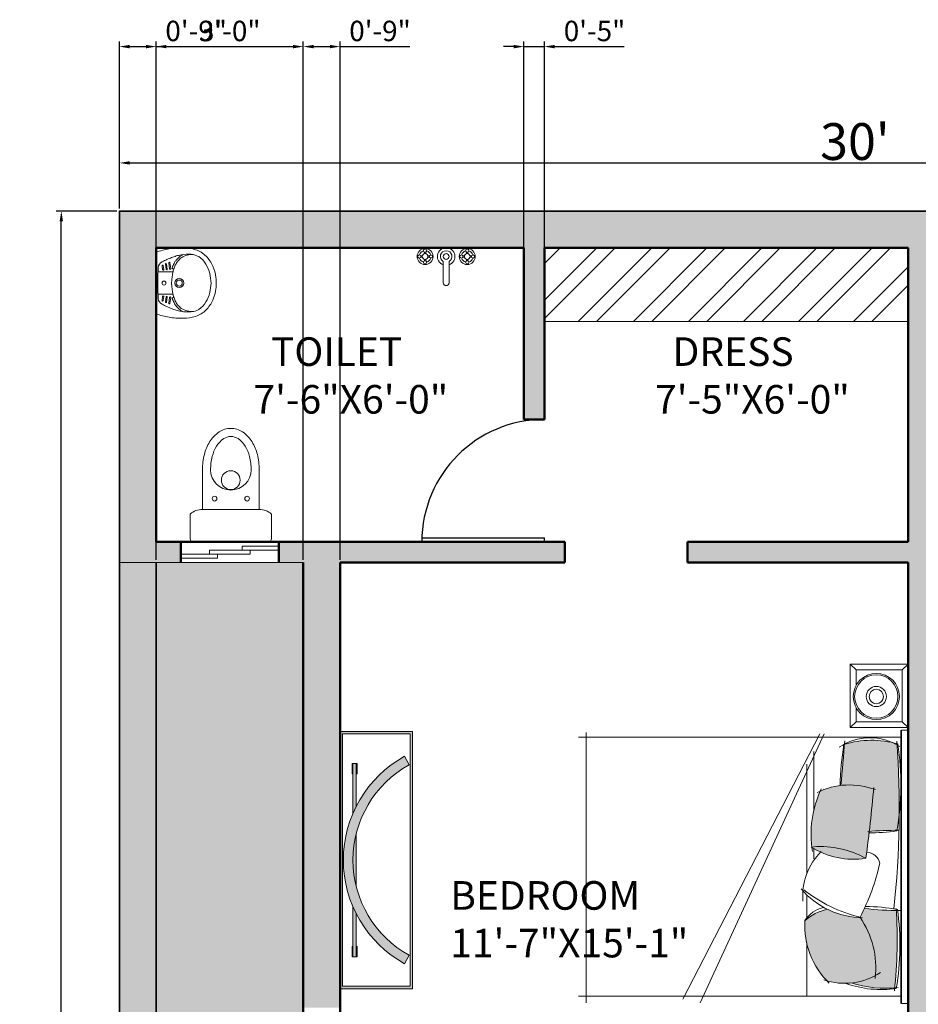
# Model space of a CAD drawing. Units: inches. Extents: x 1734 to 4011, y 1071 to 1891.
# Tile 5 of 27: x 1734 to 1954, y 1650 to 1891. Entities that reach past the tile are written whole.
import ezdxf

# ---------------------------------------------------------------- set-up
doc = ezdxf.new("R2010")
doc.units = ezdxf.units.IN
for name, color, linetype, lineweight in [('0.10', 252, 'Continuous', 9), ('0.15', 34, 'Continuous', 15), ('A-ANNO-DIMS', 2, 'Continuous', 18), ('A-AREA-IDEN', 3, 'Continuous', 18), ('A-DOOR', 3, 'Continuous', 25), ('A-FLOR-FIXT', 9, 'Continuous', 18), ('A-FLOR-PATT', 252, 'Continuous', 13), ('A-FURN', 8, 'Continuous', 18), ('A-FURN-PATT', 252, 'Continuous', 13), ('A-GLAZ', 4, 'Continuous', 18), ('A-WALL', 7, 'Continuous', 50), ('A-WALL-PATT', 8, 'Continuous', 13), ('aparador', 36, 'Continuous', 9), ('C-PROP', 1, 'Continuous', 35), ('moveis', 254, 'Continuous', 5)]:
    doc.layers.add(name, color=color, linetype=linetype, lineweight=lineweight)
doc.styles.get("Standard").update_dxf_attribs({"font": 'arial.ttf'})
doc.dimstyles.new('ISO-25', dxfattribs={"dimtxt": 5, "dimasz": 2.5, "dimexe": 1.25, "dimexo": 0.625, "dimtad": 1, "dimdec": 1, "dimlunit": 3, "dimtxsty": 'Standard', "dimcen": 2.5, "dimclrt": 1, "dimadec": 0, "dimazin": 0, "dimtfac": 1, "dimtdec": 1, "dimtmove": 0, "dimatfit": 3, "dimfxl": 1, "dimarcsym": 0})

# ---------------------------------------------------------------- blocks, each defined once
blk = doc.blocks.new('*D14')
at = {"layer": 'A-ANNO-DIMS', "color": 0, "lineweight": -2, "transparency": 16777216}
for p, q in [((1758.65, 1844.69), (1758.65, 1857.09)), ((1761.15, 1855.84), (2116.15, 1855.84)), ((2118.65, 1844.69), (2118.65, 1857.09))]:
    blk.add_line(p, q, dxfattribs=at)
at = {"layer": 'A-ANNO-DIMS', "color": 0, "transparency": 16777216}
for points in [[(1761.15, 1856.26), (1761.15, 1855.43), (1758.65, 1855.84)], [(2116.15, 1856.26), (2116.15, 1855.43), (2118.65, 1855.84)]]:
    blk.add_solid(points, dxfattribs=at)
at = {"layer": 'Defpoints', "color": 0, "transparency": 16777216}
for p in [(2118.65, 1855.84), (1758.65, 1844.06), (2118.65, 1844.06)]:
    blk.add_point(p, dxfattribs=at)
at = {"layer": 'A-ANNO-DIMS', "color": 0, "transparency": 16777216, "insert": (1938.65, 1861.07), "char_height": 5, "attachment_point": 5}
blk.add_mtext("{\\H1.8x;30'}", dxfattribs=at)
blk = doc.blocks.new('*D15')
at = {"layer": 'A-ANNO-DIMS', "color": 0, "lineweight": -2, "transparency": 16777216}
for p, q in [((1758.02, 1844.06), (1743.18, 1844.06)), ((1744.43, 1126.56), (1744.43, 1841.56)), ((1758.02, 1124.06), (1743.18, 1124.06))]:
    blk.add_line(p, q, dxfattribs=at)
at = {"layer": 'A-ANNO-DIMS', "color": 0, "transparency": 16777216}
for points in [[(1744.01, 1841.56), (1744.84, 1841.56), (1744.43, 1844.06)], [(1744.01, 1126.56), (1744.84, 1126.56), (1744.43, 1124.06)]]:
    blk.add_solid(points, dxfattribs=at)
at = {"layer": 'Defpoints', "color": 0, "transparency": 16777216}
for p in [(1744.43, 1844.06), (1758.65, 1844.06), (1758.65, 1124.06)]:
    blk.add_point(p, dxfattribs=at)
at = {"layer": 'A-ANNO-DIMS', "color": 0, "transparency": 16777216, "insert": (1739.21, 1484.06), "char_height": 5, "attachment_point": 5, "rotation": 90}
blk.add_mtext("{\\H1.8x;60'}", dxfattribs=at)
blk = doc.blocks.new("D2 2'6")
for p, q in [((0, 30), (0, 0)), ((1, 30), (1, 0)), ((0, 0), (1, 0))]:
    blk.add_line(p, q)
blk.add_arc((0, 0), 30, 0, 90)
blk = doc.blocks.new('camita')
at = {"layer": '0.10'}
for p, q in [((-0.85, -0.045), (0.85, -0.045)), ((-0.805, -0.045), (-0.805, -2.0485)), ((0.805, -0.045), (0.805, -2.0485)), ((-0.8271, -0.521), (0.8464, -1.2932)), ((-0.8271, -0.5476), (0.8236, -1.3992)), ((-0.7161, -0.585), (-0.3554, -0.585)), ((-0.1136, -0.585), (-0.0485, -0.585)), ((-0.638, -0.63), (0.0434, -0.63)), ((0.1749, -0.63), (0.3179, -0.63)), ((0.4739, -0.63), (0.805, -0.63)), ((-0.8354, -2), (0.8464, -2))]:
    blk.add_line(p, q, dxfattribs=at)
blk.add_lwpolyline([(-0.85, -0.0405), (0.85, -0.0405), (0.85, 0), (-0.85, 0)], close=True, dxfattribs=at)
for centre, radius, start, end in [((-0.4574, -0.2364), 0.3443, 147.50996, 213.83359), ((-0.3639, -5.8457), 5.7909, 83.80731, 94.12107), ((-0.5104, -1.7232), 1.6781, 80.12554, 98.66187), ((2.3534, -0.0532), 2.5803, 180.10628, 184.38541), ((-1.4396, -0.0609), 1.7117, 352.92911, 0.39592), ((0.4863, -1.6286), 1.5781, 80.16015, 98.05996), ((-0.1997, -0.2266), 0.5864, 163.92635, 197.14087), ((-1.5443, -0.2452), 1.3333, 359.93941, 7.55329), ((1.5815, -0.2893), 1.3353, 170.38021, 178.99138), ((0.4524, -3.0675), 2.9996, 83.90257, 93.67595), ((0.0294, -0.1377), 0.7262, 342.58415, 6.00484), ((0.1326, -0.1696), 0.6307, 339.92303, 8.74334), ((-0.007, -0.258), 0.0828, 100.01798, 179.73597), ((-0.2931, -1.4378), 1.2903, 61.97485, 77.84351), ((0.3203, -0.3944), 0.4043, 341.45245, 33.45121), ((-0.0543, -0.3633), 0.4542, 159.30257, 206.50263), ((-1.3301, -9.6748), 9.4985, 82.27078, 84.93989), ((0.6265, -0.7518), 0.5508, 82.96906, 124.67388), ((0.4585, -0.5454), 0.5842, 151.04555, 184.14969), ((-0.5341, -0.3393), 0.4875, 327.26442, 9.0473), ((-0.1986, -0.2742), 0.5159, 310.73945, 359.05759), ((-0.5673, -0.0868), 0.9057, 321.69527, 346.46261), ((-1.8672, -14.986), 14.6323, 84.65974, 85.75157), ((-0.4598, 1.4861), 1.9092, 260.95299, 268.65169), ((-0.2002, 0.064), 0.6673, 244.78094, 279.06058), ((0.179, -0.272), 0.3828, 224.52836, 275.22287), ((0.4384, -0.4834), 0.1898, 193.68485, 236.70352), ((0.5707, -0.4317), 0.3145, 192.93877, 221.96363), ((0.3612, -0.133), 0.5096, 267.25889, 315.29965)]:
    blk.add_arc(centre, radius, start, end, dxfattribs=at)
blk = doc.blocks.new('VELADOR')
at = {"layer": '0.15'}
for p, q in [((-0.2475, 0), (-0.2025, -0.045)), ((0.2475, 0), (0.2025, -0.045)), ((-0.2025, -0.405), (-0.2475, -0.45)), ((0.2475, -0.45), (0.2025, -0.405))]:
    blk.add_line(p, q, dxfattribs=at)
blk.add_lwpolyline([(-0.2475, 0), (-0.2475, -0.45), (0.2475, -0.45), (0.2475, 0)], close=True, dxfattribs=at)
blk.add_lwpolyline([(0.0921, -0.405), (0.2025, -0.405), (0.2025, -0.045), (-0.2025, -0.045), (-0.2025, -0.405), (-0.0818, -0.405)], dxfattribs=at)
for radius in [0.18, 0.1688, 0.0788, 0.0563]:
    blk.add_circle((0.0052, -0.2474), radius, dxfattribs=at)
blk = doc.blocks.new('Aparador ORGANICA Formatto')
at = {"layer": 'aparador', "ltscale": 0.3}
h = blk.add_hatch(color=256, dxfattribs=at)
h.dxf.hatch_style = 1
h.set_gradient(color1=(118, 213, 123), color2=(52, 168, 57), one_color=1, tint=0.43, name='INVCURVED')
h.paths.add_polyline_path([(0.8, 0.45), (-0.8, 0.45), (-0.8, 0), (0.8, 0)])
h.paths.add_polyline_path([(0.785, 0.435), (0.785, 0.015), (-0.785, 0.015), (-0.785, 0.435)], flags=16)
h.paths.add_polyline_path([(0.2911, 0.3699), (0.5365, 0.3699), (0.5365, 0.3757), (0.6011, 0.3757), (0.6011, 0.3699), (0.6011, 0.3499), (0.6011, 0.3441), (0.5365, 0.3441), (0.5365, 0.3499), (0.3338, 0.3499, -0.150336), (0.6449, 0.0488), (0.5923, 0.0199, 0.208852), (0.1632, 0.3499), (-0.1632, 0.3499, 0.208852), (-0.5923, 0.0199), (-0.6449, 0.0488, -0.150336), (-0.3338, 0.3499), (-0.5365, 0.3499), (-0.5365, 0.3441), (-0.6011, 0.3441), (-0.6011, 0.3499), (-0.6011, 0.3699), (-0.6011, 0.3757), (-0.5365, 0.3757), (-0.5365, 0.3699), (-0.2911, 0.3699, -0.206106)], flags=0)
h = blk.add_hatch(color=256, dxfattribs=at)
h.dxf.hatch_style = 1
h.set_gradient(color1=(135, 92, 69), color2=(0, 0, 0), one_color=1, name='INVCURVED')
h.paths.add_polyline_path([(-0.6449, 0.0488), (-0.5923, 0.0199, -0.590888), (0.5923, 0.0199), (0.6449, 0.0488, 0.590888)])
h = blk.add_hatch(color=256, dxfattribs=at)
h.dxf.hatch_style = 1
h.set_gradient(color1=(178, 189, 189), one_color=1, tint=1, name='CYLINDER')
h.paths.add_polyline_path([(-0.5365, 0.3757), (-0.6011, 0.3757), (-0.6011, 0.3699), (-0.5365, 0.3699)])
h.paths.add_polyline_path([(-0.5365, 0.3499), (-0.6011, 0.3499), (-0.6011, 0.3441), (-0.5365, 0.3441)])
h = blk.add_hatch(color=256, dxfattribs=at)
h.dxf.hatch_style = 1
h.set_gradient(color1=(118, 213, 123), color2=(31, 101, 35), one_color=1, tint=0.26, name='INVCURVED')
h.paths.add_polyline_path([(-0.2911, 0.3699), (-0.6011, 0.3699), (-0.6011, 0.3499), (-0.3338, 0.3499, -0.015999)])
h = blk.add_hatch(color=256, dxfattribs=at)
h.dxf.hatch_style = 1
h.set_gradient(color1=(118, 213, 123), color2=(31, 101, 35), one_color=1, tint=0.26, name='INVCURVED')
h.paths.add_polyline_path([(-0.1632, 0.3499), (0.1632, 0.3499, 0.122516)])
h = blk.add_hatch(color=256, dxfattribs=at)
h.dxf.hatch_style = 1
h.set_gradient(color1=(118, 213, 123), color2=(31, 101, 35), one_color=1, tint=0.26, name='INVCURVED')
h.paths.add_polyline_path([(0.6011, 0.3699), (0.2911, 0.3699, -0.015999), (0.3338, 0.3499), (0.6011, 0.3499)])
h = blk.add_hatch(color=256, dxfattribs=at)
h.dxf.hatch_style = 1
h.set_gradient(color1=(178, 189, 189), one_color=1, tint=1, name='CYLINDER')
h.paths.add_polyline_path([(0.6011, 0.3757), (0.5365, 0.3757), (0.5365, 0.3699), (0.6011, 0.3699)])
h.paths.add_polyline_path([(0.6011, 0.3499), (0.5365, 0.3499), (0.5365, 0.3441), (0.6011, 0.3441)])
for p, q in [((-0.5923, 0.0199), (-0.6449, 0.0488)), ((0.5923, 0.0199), (0.6449, 0.0488))]:
    blk.add_line(p, q, dxfattribs=at)
for points in [[(-0.6011, 0.3699), (-0.6011, 0.3757), (-0.5365, 0.3757), (-0.5365, 0.3699)], [(0.6011, 0.3699), (0.6011, 0.3757), (0.5365, 0.3757), (0.5365, 0.3699)], [(-0.5365, 0.3499), (-0.5365, 0.3441), (-0.6011, 0.3441), (-0.6011, 0.3499)], [(0.5365, 0.3499), (0.5365, 0.3441), (0.6011, 0.3441), (0.6011, 0.3499)]]:
    blk.add_lwpolyline(points, dxfattribs=at)
for radius in [0.7362, 0.6762]:
    blk.add_arc((0, -0.3063), radius, 28.84335, 151.15665, dxfattribs=at)
at = {"layer": 'moveis', "ltscale": 0.3}
for p, q in [((-0.6011, 0.3699), (-0.6011, 0.3499)), ((-0.2911, 0.3699), (-0.6011, 0.3699)), ((0.2911, 0.3699), (0.6011, 0.3699)), ((0.6011, 0.3699), (0.6011, 0.3499)), ((-0.6011, 0.3499), (-0.3338, 0.3499)), ((-0.1632, 0.3499), (0.1632, 0.3499)), ((0.6011, 0.3499), (0.3338, 0.3499))]:
    blk.add_line(p, q, dxfattribs=at)
for points in [[(-0.8, 0), (0.8, 0), (0.8, 0.45), (-0.8, 0.45)], [(-0.785, 0.015), (0.785, 0.015), (0.785, 0.435), (-0.785, 0.435)]]:
    blk.add_lwpolyline(points, close=True, dxfattribs=at)
blk = doc.blocks.new('Faucet - Bathroom top')
for p, q in [((-4.107, 0.125), (-4.375, 0.125)), ((-3.75, 0.4788), (-3.75, 0.75)), ((-3.5, 0.482), (-3.5, 0.75)), ((-3.1461, 0.125), (-2.875, 0.125)), ((3.143, 0.125), (2.875, 0.125)), ((3.5, 0.4788), (3.5, 0.75)), ((3.75, 0.482), (3.75, 0.75)), ((4.1039, 0.125), (4.375, 0.125)), ((-4.1039, -0.125), (-4.375, -0.125)), ((-3.75, -0.4821), (-3.75, -0.75)), ((-3.5, -0.4789), (-3.5, -0.75)), ((-3.143, -0.125), (-2.875, -0.125)), ((-0.5, -0.8639), (-0.5, -4.5)), ((0.5, -4.5), (0.5, -0.8631)), ((3.1461, -0.125), (2.875, -0.125)), ((3.5, -0.4821), (3.5, -0.75)), ((3.75, -0.4789), (3.75, -0.75)), ((4.107, -0.125), (4.375, -0.125))]:
    blk.add_line(p, q)
for centre, radius in [((-3.625, 0), 1.375), ((-4.625, 0), 0.2795), ((-3.625, 0), 0.5), ((-3.625, 1), 0.2795), ((-2.625, 0), 0.2795), ((0, 0), 0.5), ((3.625, 0), 1.375), ((2.625, 0), 0.2795), ((3.625, 0), 0.5), ((3.625, 1), 0.2795), ((4.625, 0), 0.2795), ((-3.625, -1), 0.2795), ((3.625, -1), 0.2795)]:
    blk.add_circle(centre, radius)
for centre, radius, start, end in [((-3.625, 0), 1, 105.2407, 164.2093), ((-3.625, 0), 1, 16.44125, 74.07887), ((0, 0), 1.5, 289.6514, 250.3603), ((0, 0), 1, 300.3431, 239.7554), ((3.625, 0), 1, 106.12, 164.0884), ((3.625, 0), 1, 16.23422, 73.90469), ((-3.625, 0), 1, 196.2342, 253.9047), ((-3.625, 0), 1, 286.12, 344.0884), ((3.625, 0), 1, 196.4413, 254.0789), ((3.625, 0), 1, 285.2407, 344.2093), ((0, -4.5), 0.5, 180, 0)]:
    blk.add_arc(centre, radius, start, end)
blk = doc.blocks.new('lavamanos 2')
at = {"layer": '0.15'}
for p, q in [((0, 0.2335), (0, -0.2335)), ((-0.1127, 0.112), (-0.1067, 0.1581)), ((-0.1037, 0.1109), (-0.0978, 0.157)), ((-0.1304, 0.11), (-0.1315, 0.11)), ((-0.0142, 0.087), (-0.13, 0.086)), ((-0.0857, 0.1085), (-0.0807, 0.1466)), ((-0.0767, 0.1074), (-0.0718, 0.1455)), ((-0.0587, 0.105), (-0.0548, 0.1351)), ((-0.0497, 0.1039), (-0.0458, 0.134)), ((-0.1304, -0.11), (-0.1315, -0.11)), ((-0.0142, -0.087), (-0.13, -0.086)), ((-0.1127, -0.112), (-0.1067, -0.1581)), ((-0.1037, -0.1109), (-0.0978, -0.157)), ((-0.0857, -0.1085), (-0.0807, -0.1466)), ((-0.0767, -0.1074), (-0.0718, -0.1455)), ((-0.0587, -0.105), (-0.0548, -0.1351)), ((-0.0497, -0.1039), (-0.0458, -0.134))]:
    blk.add_line(p, q, dxfattribs=at)
for centre, radius in [((-0.178, 0), 0.035), ((-0.178, 0), 0.0235), ((-0.06, 0), 0.015)]:
    blk.add_circle(centre, radius, dxfattribs=at)
for centre, radius, start, end in [((-0.2419, 0.0663), 0.2023, 108.1945, 135.36859), ((-0.2035, -0.0862), 0.3593, 91.20299, 106.42552), ((-0.2208, -0.6855), 0.9585, 86.55138, 89.41308), ((-0.2121, -0.5476), 0.8204, 83.12241, 86.5796), ((5.8279, 30.215), 30.5319, 258.77821, 258.87599), ((-0.1265, -0.0657), 0.3287, 69.06009, 78.82181), ((-0.0202, 0.212), 0.0314, 54.79491, 69.06009), ((-0.005, 0.2335), 0.005, 0, 54.79491), ((-0.1663, 0.0005), 0.3024, 136.57187, 154.32772), ((-0.2422, 0.0655), 0.1638, 121.99295, 150.58892), ((-0.2657, 0.1037), 0.119, 92.47742, 122.14108), ((-0.2765, 0.0677), 0.1528, 57.2491, 95.54005), ((-0.2442, -0.0128), 0.2368, 77.24819, 96.46321), ((-0.2765, 0.0677), 0.1678, 56.87663, 64.99714), ((-0.3662, -0.002), 0.2627, 40.35252, 49.00458), ((-0.2222, 0.0026), 0.2177, 71.98488, 82.01242), ((-0.3662, -0.002), 0.2777, 40.35252, 49.22548), ((-0.2374, 0.11), 0.0921, 27.31862, 39.11562), ((-0.3103, -0.315), 0.5472, 69.51913, 73.49118), ((-0.2374, 0.11), 0.1071, 27.57433, 39.11562), ((-0.3494, 0.0363), 0.2408, 22.19214, 30.78376), ((-0.2991, -0.2855), 0.5156, 65.23004, 69.53785), ((-0.1022, 0.1575), 0.0045, 352.61396, 172.61396), ((-0.2784, -0.2408), 0.4663, 60.24131, 65.2382), ((-0.0648, 0.1184), 0.049, 1.58272, 68.62081), ((-0.0557, -0.0178), 0.4111, 158.70106, 171.31016), ((-0.1999, 0.0263), 0.2202, 147.11565, 167.44248), ((-0.3494, 0.0363), 0.2258, 22.33605, 30.8927), ((-1.2664, -0.2389), 1.1824, 16.36313, 17.77674), ((-0.1315, 0.117), 0.007, 197.40991, 270.49494), ((0.1853, 0.1648), 0.325, 192.53887, 196.70718), ((-0.1305, 0.117), 0.007, 270.49494, 17.39527), ((-1.2664, -0.2389), 1.1974, 17.39527, 17.80495), ((-0.1082, 0.1115), 0.0045, 172.61396, 352.61396), ((-0.0812, 0.108), 0.0045, 172.61396, 352.61396), ((-0.0763, 0.146), 0.0045, 352.61396, 172.61396), ((-0.0542, 0.1045), 0.0045, 172.61396, 352.61396), ((-0.0503, 0.1345), 0.0045, 352.61396, 172.61396), ((-2.1477, 0.0009), 2.1352, 359.97535, 3.19009), ((-0.2093, 0.0056), 0.2558, 171.31016, 181.26266), ((-0.2093, -0.0056), 0.2558, 178.73734, 188.68984), ((0.4664, -0.0834), 0.8953, 169.86317, 174.65802), ((0.4664, 0.0834), 0.8953, 185.34198, 190.13683), ((0.3887, 0.121), 0.517, 185.50529, 189.81306), ((-0.7181, -0.0071), 0.5987, 0.67647, 3.82165), ((-0.7181, 0.0071), 0.5987, 356.17835, 359.32353), ((-2.1477, -0.0009), 2.1352, 356.80991, 0.02465), ((-0.0557, 0.0178), 0.4111, 188.68984, 201.29894), ((-0.1999, -0.0263), 0.2202, 192.55752, 212.88435), ((0.1853, -0.1648), 0.325, 163.29282, 167.46113), ((0.3887, -0.1209), 0.517, 170.18694, 174.49471), ((-0.1663, -0.0005), 0.3024, 205.67228, 223.42813), ((-0.2422, -0.0655), 0.1638, 209.41108, 238.00705), ((-0.2374, -0.1099), 0.0921, 320.88438, 332.68138), ((-0.3494, -0.0363), 0.2258, 329.1073, 337.66395), ((-0.3494, -0.0363), 0.2408, 329.21624, 337.80786), ((-1.2664, 0.2389), 1.1824, 342.22326, 343.63687), ((-0.1315, -0.117), 0.007, 89.50506, 162.59009), ((-0.1305, -0.117), 0.007, 342.60473, 89.50506), ((-1.2664, 0.2389), 1.1974, 342.19505, 342.60473), ((-0.1082, -0.1115), 0.0045, 7.38604, 187.38604), ((-0.0812, -0.108), 0.0045, 7.38604, 187.38604), ((-0.0763, -0.146), 0.0045, 187.38604, 7.38604), ((-0.0542, -0.1045), 0.0045, 7.38604, 187.38604), ((-0.0503, -0.1345), 0.0045, 187.38604, 7.38604), ((-0.0648, -0.1184), 0.049, 291.37919, 358.41728), ((-0.2419, -0.0663), 0.2023, 224.63141, 251.8055), ((-0.2657, -0.1036), 0.119, 237.85892, 267.52258), ((-0.2765, -0.0677), 0.1528, 264.45995, 302.7509), ((-0.2442, 0.0128), 0.2368, 263.53679, 282.75181), ((-0.2765, -0.0677), 0.1678, 295.00286, 303.12337), ((-0.3662, 0.002), 0.2627, 310.99542, 319.64748), ((-0.2222, -0.0026), 0.2177, 277.98758, 288.01512), ((-0.3662, 0.002), 0.2777, 310.77452, 319.64748), ((-0.3103, 0.315), 0.5472, 286.50882, 290.48087), ((-0.2374, -0.1099), 0.1071, 320.88438, 332.42567), ((-0.2991, 0.2855), 0.5156, 290.46215, 294.76996), ((-0.1022, -0.1575), 0.0045, 187.38604, 7.38604), ((-0.2784, 0.2408), 0.4663, 294.7618, 299.75869), ((-0.2035, 0.0862), 0.3593, 253.57448, 268.79701), ((-0.2208, 0.6855), 0.9585, 270.58692, 273.44862), ((-0.2121, 0.5476), 0.8204, 273.4204, 276.87759), ((5.8279, -30.215), 30.5319, 101.12401, 101.22179), ((-0.1265, 0.0657), 0.3287, 281.17819, 290.93991), ((-0.0202, -0.212), 0.0314, 290.93991, 305.20509), ((-0.005, -0.2335), 0.005, 305.20509, 0)]:
    blk.add_arc(centre, radius, start, end, dxfattribs=at)
blk = doc.blocks.new('rreerr')
blk.add_lwpolyline([(2512.8529, 833.5601, 0.205217), (2512.9279, 833.5883), (2512.9279, 833.7401, 0.414214), (2512.9079, 833.7601), (2512.4479, 833.7601, 0.414214), (2512.4279, 833.7401), (2512.4279, 833.5883, 0.205217), (2512.5029, 833.5601)], format="xyb")
for points in [[(2512.5468, 833.1438, 0.107027), (2512.6056, 833.0819, 0.150548), (2512.6779, 833.0596, 0.150548), (2512.7502, 833.0819, 0.107027), (2512.809, 833.1438, 0.075071), (2512.8412, 833.2206, 0.0618), (2512.8529, 833.3151), (2512.8529, 833.5601), (2512.5029, 833.5601), (2512.5029, 833.3151, 0.0618), (2512.5146, 833.2206, 0.075071)], [(2512.5631, 833.2328, 0.075071), (2512.5895, 833.1698, 0.107027), (2512.6338, 833.1232, 0.150548), (2512.6779, 833.1096, 0.150548), (2512.722, 833.1232, 0.107027), (2512.7663, 833.1698, 0.075071), (2512.7927, 833.2328, 0.0618), (2512.8029, 833.3151, 1), (2512.5529, 833.3151, 0.0618)]]:
    blk.add_lwpolyline(points, format="xyb", close=True)
for centre, radius in [((2512.5779, 833.493), 0.0146), ((2512.7779, 833.493), 0.0146), ((2512.6775, 833.3793), 0.0579)]:
    blk.add_circle(centre, radius)
blk = doc.blocks.new('*D103')
at = {"layer": 'A-ANNO-DIMS', "color": 0, "lineweight": -2, "transparency": 16777216}
for p, q in [((1758.65, 1844.69), (1758.65, 1885.56)), ((1767.65, 1835.69), (1767.65, 1885.56)), ((1761.15, 1884.31), (1765.15, 1884.31)), ((1767.65, 1884.31), (1784.69, 1884.31))]:
    blk.add_line(p, q, dxfattribs=at)
at = {"layer": 'A-ANNO-DIMS', "color": 0, "transparency": 16777216}
for points in [[(1761.15, 1884.73), (1761.15, 1883.89), (1758.65, 1884.31)], [(1765.15, 1884.73), (1765.15, 1883.89), (1767.65, 1884.31)]]:
    blk.add_solid(points, dxfattribs=at)
at = {"layer": 'Defpoints', "color": 0, "transparency": 16777216}
for p in [(1767.65, 1884.31), (1758.65, 1844.06), (1767.65, 1835.06)]:
    blk.add_point(p, dxfattribs=at)
at = {"layer": 'A-ANNO-DIMS', "color": 1, "transparency": 16777216, "insert": (1777.42, 1887.49), "char_height": 5, "attachment_point": 5}
blk.add_mtext('0\'-9"', dxfattribs=at)
blk = doc.blocks.new('*D105')
at = {"layer": 'A-ANNO-DIMS', "color": 0, "lineweight": -2, "transparency": 16777216}
for p, q in [((1857.65, 1793.69), (1857.65, 1885.56)), ((1862.65, 1793.69), (1862.65, 1885.56)), ((1855.15, 1884.31), (1852.65, 1884.31)), ((1857.65, 1884.31), (1862.65, 1884.31)), ((1865.15, 1884.31), (1882.19, 1884.31))]:
    blk.add_line(p, q, dxfattribs=at)
at = {"layer": 'A-ANNO-DIMS', "color": 0, "transparency": 16777216}
for points in [[(1855.15, 1884.73), (1855.15, 1883.89), (1857.65, 1884.31)], [(1865.15, 1884.73), (1865.15, 1883.89), (1862.65, 1884.31)]]:
    blk.add_solid(points, dxfattribs=at)
at = {"layer": 'Defpoints', "color": 0, "transparency": 16777216}
for p in [(1862.65, 1884.31), (1857.65, 1793.06), (1862.65, 1793.06)]:
    blk.add_point(p, dxfattribs=at)
at = {"layer": 'A-ANNO-DIMS', "color": 1, "transparency": 16777216, "insert": (1874.92, 1887.49), "char_height": 5, "attachment_point": 5}
blk.add_mtext('0\'-5"', dxfattribs=at)
blk = doc.blocks.new('*D106')
at = {"layer": 'A-ANNO-DIMS', "color": 0, "lineweight": -2, "transparency": 16777216}
for p, q in [((1767.65, 1758.69), (1767.65, 1885.56)), ((1803.65, 1758.69), (1803.65, 1885.56)), ((1770.15, 1884.31), (1801.15, 1884.31))]:
    blk.add_line(p, q, dxfattribs=at)
at = {"layer": 'A-ANNO-DIMS', "color": 0, "transparency": 16777216}
for points in [[(1770.15, 1884.73), (1770.15, 1883.89), (1767.65, 1884.31)], [(1801.15, 1884.73), (1801.15, 1883.89), (1803.65, 1884.31)]]:
    blk.add_solid(points, dxfattribs=at)
at = {"layer": 'Defpoints', "color": 0, "transparency": 16777216}
for p in [(1803.65, 1884.31), (1767.65, 1758.06), (1803.65, 1758.06)]:
    blk.add_point(p, dxfattribs=at)
at = {"layer": 'A-ANNO-DIMS', "color": 1, "transparency": 16777216, "insert": (1785.65, 1887.49), "char_height": 5, "attachment_point": 5}
blk.add_mtext('3\'-0"', dxfattribs=at)
blk = doc.blocks.new('*D107')
at = {"layer": 'A-ANNO-DIMS', "color": 0, "lineweight": -2, "transparency": 16777216}
for p, q in [((1803.65, 1758.69), (1803.65, 1885.56)), ((1812.65, 1758.69), (1812.65, 1885.56)), ((1806.15, 1884.31), (1810.15, 1884.31)), ((1812.65, 1884.31), (1829.69, 1884.31))]:
    blk.add_line(p, q, dxfattribs=at)
at = {"layer": 'A-ANNO-DIMS', "color": 0, "transparency": 16777216}
for points in [[(1806.15, 1884.73), (1806.15, 1883.89), (1803.65, 1884.31)], [(1810.15, 1884.73), (1810.15, 1883.89), (1812.65, 1884.31)]]:
    blk.add_solid(points, dxfattribs=at)
at = {"layer": 'Defpoints', "color": 0, "transparency": 16777216}
for p in [(1812.65, 1884.31), (1803.65, 1758.06), (1812.65, 1758.06)]:
    blk.add_point(p, dxfattribs=at)
at = {"layer": 'A-ANNO-DIMS', "color": 1, "transparency": 16777216, "insert": (1822.42, 1887.49), "char_height": 5, "attachment_point": 5}
blk.add_mtext('0\'-9"', dxfattribs=at)

msp = doc.modelspace()

# ---------------------------------------------------------------- hatches: boundary and pattern name
at = {"layer": 'A-FLOR-PATT'}
h = msp.add_hatch(color=256, dxfattribs=at)
h.dxf.hatch_style = 1
h.paths.add_polyline_path([(1767.65, 1758.06), (1758.65, 1758.06), (1758.65, 1124.06), (1814.65, 1124.06), (1814.65, 1133.06), (1767.65, 1133.06)])
h = msp.add_hatch(color=256, dxfattribs=at)
h.dxf.hatch_style = 1
h.paths.add_polyline_path([(1803.65, 1758.06), (1767.65, 1758.06), (1767.65, 1325.06), (1803.65, 1325.06), (1803.65, 1542.06)])
at = {"layer": 'A-FURN-PATT'}
h = msp.add_hatch(dxfattribs=at)
h.set_pattern_fill('ANSI32', color=256)
h.paths.add_polyline_path([(1951.65, 1835.06), (1862.65, 1835.06), (1862.65, 1817.06), (1951.65, 1817.06)])
h.paths.add_polyline_path([(1896.65, 1466.06), (1812.65, 1466.06), (1812.65, 1448.06), (1896.65, 1448.06)])
h.paths.add_polyline_path([(1826.14, 1452.28), (1875.6, 1452.28), (1875.6, 1462.58), (1826.14, 1462.58)], flags=24)
h = msp.add_hatch(color=256, dxfattribs=at)
h.dxf.hatch_style = 1
h.paths.add_polyline_path([(1948.97, 1713.4, 0.020657), (1947.97, 1713.91, 0.131047), (1936.07, 1713.53, -0.004387), (1935.22, 1703.46, -0.113891), (1943.22, 1702.59, -0.006967), (1942.14, 1692.22, -0.016701), (1948.92, 1692.49, 0.015442), (1949.49, 1696.53, 0.01851)])
h.paths.add_polyline_path([(1948.76, 1672.85, -0.029051), (1940.95, 1673.36, -0.011742), (1939.88, 1671.23, -0.175864), (1943.64, 1656.92, -0.098488), (1937.7, 1655.11, 0.094792), (1948.38, 1653.89, 0.040212)])
h = msp.add_hatch(color=256, dxfattribs=at)
h.dxf.hatch_style = 1
h.paths.add_polyline_path([(1943.22, 1702.59, 0.189536), (1930.14, 1702.07, 0.134508), (1928.08, 1688.34, 0.181694), (1941.31, 1685.63, 0.011408)])
h.paths.add_polyline_path([(1939.98, 1671.09, -0.104045), (1931.88, 1673.16, 0.127326), (1926.37, 1670.3, 0.202559), (1931.75, 1655.64, 0.194952), (1943.64, 1656.92, 0.173835)])
at = {"layer": 'A-WALL-PATT'}
h = msp.add_hatch(color=256, dxfattribs=at)
h.dxf.hatch_style = 1
h.paths.add_polyline_path([(1857.65, 1835.06), (1857.65, 1793.06), (1862.65, 1793.06), (1862.65, 1835.06), (1951.65, 1835.06), (1951.65, 1763.06), (1897.65, 1763.06), (1897.65, 1758.06), (1951.65, 1758.06), (1951.65, 1617.06), (1956.65, 1617.06), (1956.65, 1758.06), (2009.65, 1758.06), (2009.65, 1763.06), (1956.65, 1763.06), (1956.65, 1835.06), (2044.65, 1835.06), (2044.65, 1763.06), (2039.65, 1763.06), (2039.65, 1758.06), (2054.65, 1758.06), (2054.65, 1763.06), (2049.65, 1763.06), (2049.65, 1835.06), (2109.65, 1835.06), (2109.65, 1763.06), (2084.65, 1763.06), (2084.65, 1758.06), (2109.65, 1758.06), (2109.65, 1530.06), (2095.15, 1530.06), (2095.15, 1525.06), (2109.65, 1525.06), (2109.65, 1471.06), (2089.15, 1471.06), (2089.15, 1466.06), (2109.65, 1466.06), (2109.65, 1250.06), (2015.65, 1250.06), (2015.65, 1241.06), (2109.65, 1241.06), (2109.65, 1133.06), (1952.65, 1133.06), (1952.65, 1197.06), (1953.65, 1197.06), (1953.65, 1202.06), (1946.65, 1202.06), (1946.65, 1133.06), (1934.65, 1133.06), (1934.65, 1124.06), (2118.65, 1124.06), (2118.65, 1844.06), (1758.65, 1844.06), (1758.65, 1758.06), (1773.65, 1758.06), (1773.65, 1763.06), (1767.65, 1763.06), (1767.65, 1835.06)])
h.paths.add_polyline_path([(1803.65, 1649.06), (1812.65, 1649.06), (1812.65, 1758.06), (1867.65, 1758.06), (1867.65, 1763.06), (1797.65, 1763.06), (1797.65, 1758.06), (1803.65, 1758.06)], flags=17)
h.paths.add_polyline_path([(1803.65, 1572.06), (1956.65, 1572.06), (1956.65, 1581.06), (1951.65, 1581.06), (1951.65, 1577.06), (1812.65, 1577.06), (1812.65, 1601.06), (1803.65, 1601.06)], flags=17)
h.paths.add_polyline_path([(2044.65, 1530.06), (2044.65, 1525.06), (2059.15, 1525.06), (2059.15, 1530.06)], flags=17)
h.paths.add_polyline_path([(2009.65, 1466.06), (2035.15, 1466.06), (2035.15, 1471.06), (2014.65, 1471.06), (2014.65, 1530.06), (2009.65, 1530.06)], flags=17)
h.paths.add_polyline_path([(1896.65, 1537.06), (1896.65, 1533.06), (1901.65, 1533.06), (1901.65, 1542.06), (1803.65, 1542.06), (1803.65, 1507.06), (1812.65, 1507.06), (1812.65, 1537.06)], flags=17)
h.paths.add_polyline_path([(1906.65, 1466.06), (1906.65, 1471.06), (1901.65, 1471.06), (1901.65, 1503.06), (1896.65, 1503.06), (1896.65, 1471.06), (1812.65, 1471.06), (1812.65, 1483.06), (1803.65, 1483.06), (1803.65, 1400.06), (1812.65, 1400.06), (1812.65, 1466.06)], flags=17)
h.paths.add_polyline_path([(1951.65, 1334.06), (1909.15, 1334.06), (1909.15, 1325.06), (1956.65, 1325.06), (1956.65, 1466.06), (1961.65, 1466.06), (1961.65, 1471.06), (1942.65, 1471.06), (1942.65, 1466.06), (1951.65, 1466.06)], flags=17)
h.paths.add_polyline_path([(1812.65, 1334.06), (1812.65, 1352.06), (1803.65, 1352.06), (1803.65, 1325.06), (1855.15, 1325.06), (1855.15, 1334.06)], flags=17)
h.paths.add_polyline_path([(1956.65, 1298.06), (1956.65, 1301.06), (1947.65, 1301.06), (1947.65, 1298.06)], flags=17)
h.paths.add_polyline_path([(1967.65, 1241.06), (1967.65, 1250.06), (1947.65, 1250.06), (1947.65, 1241.06)], flags=17)

# ---------------------------------------------------------------- linework, layer by layer
at = {"layer": 'A-FURN'}
for p, q in [((1862.65, 1817.06), (1951.65, 1817.06)), ((1758.65, 1758.06), (1803.65, 1758.06))]:
    msp.add_line(p, q, dxfattribs=at)
at = {"layer": 'A-GLAZ'}
for p, q in [((1788.65, 1762.06), (1788.65, 1761.06)), ((1797.65, 1762.06), (1788.65, 1762.06)), ((1790.65, 1760.06), (1773.65, 1760.06)), ((1780.65, 1761.06), (1780.65, 1760.06)), ((1797.65, 1761.06), (1780.65, 1761.06)), ((1782.65, 1760.06), (1782.65, 1759.06)), ((1790.65, 1761.06), (1790.65, 1760.06)), ((1782.65, 1759.06), (1773.65, 1759.06))]:
    msp.add_line(p, q, dxfattribs=at)
at = {"layer": 'A-WALL'}
for p, q in [((1767.65, 1835.06), (1857.65, 1835.06)), ((1767.65, 1763.06), (1767.65, 1835.06)), ((1857.65, 1793.06), (1857.65, 1835.06)), ((1862.65, 1793.06), (1862.65, 1835.06)), ((1862.65, 1835.06), (1951.65, 1835.06)), ((1951.65, 1763.06), (1951.65, 1835.06)), ((1857.65, 1793.06), (1862.65, 1793.06)), ((1767.65, 1763.06), (1867.65, 1763.06)), ((1773.65, 1763.06), (1773.65, 1758.06)), ((1797.65, 1763.06), (1797.65, 1758.06)), ((1867.65, 1758.06), (1867.65, 1763.06)), ((1897.65, 1758.06), (1897.65, 1763.06)), ((1897.65, 1763.06), (1951.65, 1763.06)), ((1803.65, 1542.06), (1803.65, 1758.06)), ((1812.65, 1577.06), (1812.65, 1758.06)), ((1812.65, 1758.06), (1867.65, 1758.06)), ((1897.65, 1758.06), (1951.65, 1758.06)), ((1951.65, 1617.06), (1951.65, 1758.06))]:
    msp.add_line(p, q, dxfattribs=at)
at = {"layer": 'C-PROP'}
msp.add_line((1767.65, 1133.06), (1767.65, 1758.06), dxfattribs=at)
msp.add_lwpolyline([(1814.65, 1124.06), (1758.65, 1124.06), (1758.65, 1844.06), (2118.65, 1844.06), (2118.65, 1124.06), (1934.65, 1124.06)], dxfattribs=at)

# ---------------------------------------------------------------- block references
at = {"layer": 'A-DOOR', "rotation": 90.00000000000003}
msp.add_blockref("D2 2'6", (1862.65, 1763.06), dxfattribs=at)
at = {"layer": 'A-FLOR-FIXT'}
for name, p, xscale, yscale, zscale, rotation in [('lavamanos 2', (1767.65, 1826.43), 31.61240364394164, 31.61240364394164, 31.61240364394164, 179.99990349049), ('rreerr', (-97969.91, 34864.17), -39.701, 39.701, 39.701, 180)]:
    msp.add_blockref(name, p, dxfattribs=dict(at, xscale=xscale, yscale=yscale, zscale=zscale, rotation=rotation))
at = {"layer": 'A-FLOR-FIXT', "xscale": 1.424049708253414, "yscale": 1.424049708253414, "zscale": 1.424049708253414}
msp.add_blockref('Faucet - Bathroom top', (1838.61, 1832.93), dxfattribs=at)
at = {"layer": 'A-FURN'}
for name, p, xscale, yscale, zscale, rotation in [('VELADOR', (1951.65, 1725.39), 31.41542173157097, 31.41542173157097, 31.41542173157097, 270), ('Aparador ORGANICA Formatto', (1830.37, 1685.2), 39.3701, 39.3701, 39.3701, 90), ('camita', (1951.65, 1683.56), 39.375, 39.375, 39.375, 270)]:
    msp.add_blockref(name, p, dxfattribs=dict(at, xscale=xscale, yscale=yscale, zscale=zscale, rotation=rotation))

# ---------------------------------------------------------------- texts
at = {"layer": 'A-AREA-IDEN', "char_height": 7, "attachment_point": 1}
for s, heights, insert in [('  TOILET\\P7\'-6"X6\'-0"', [18.94], (1791.46, 1813.15)), ('  DRESS\\P7\'-5"X6\'-0"', [18.94], (1889.72, 1813.15)), ('BEDROOM\\P11\'-7"X15\'-1"', [0], (1839.61, 1680.04))]:
    msp.add_mtext_dynamic_manual_height_columns(s, width=86.9528, gutter_width=12.5, heights=heights, dxfattribs=dict(at, insert=insert))

# ---------------------------------------------------------------- dimensions: what is measured, and where the dimension line sits
at = {"layer": 'A-ANNO-DIMS'}
for base, p1, p2, picture, middle in [((1767.65, 1884.31), (1758.65, 1844.06), (1767.65, 1835.06), '*D103', (1777.42, 1887.49)), ((1803.65, 1884.31), (1767.65, 1758.06), (1803.65, 1758.06), '*D106', (1785.65, 1887.49)), ((1812.65, 1884.31), (1803.65, 1758.06), (1812.65, 1758.06), '*D107', (1822.42, 1887.49)), ((1862.65, 1884.31), (1857.65, 1793.06), (1862.65, 1793.06), '*D105', (1874.92, 1887.49))]:
    dim = msp.add_linear_dim(base=base, p1=p1, p2=p2, dimstyle='ISO-25', override={"dimdec": 1, "dimlfac": 1, "dimrnd": 0, "dimzin": 1, "dimdsep": 46, "dimlunit": 4, "dimfrac": 2}, dxfattribs=at)
    dim.commit()
    dim.dimension.update_dxf_attribs({"geometry": picture, "text_midpoint": middle})
dim = msp.add_linear_dim(base=(2118.65, 1855.84), p1=(1758.65, 1844.06), p2=(2118.65, 1844.06), text='{\\H1.8x;<>}', dimstyle='ISO-25', override={"dimclrd": 0, "dimclre": 0, "dimclrt": 0}, dxfattribs=at)
dim.commit()
dim.dimension.update_dxf_attribs({"geometry": '*D14', "text_midpoint": (1938.65, 1861.07)})
dim = msp.add_linear_dim(base=(1744.43, 1844.06), p1=(1758.65, 1124.06), p2=(1758.65, 1844.06), angle=90, text='{\\H1.8x;<>}', dimstyle='ISO-25', override={"dimclrd": 0, "dimclre": 0, "dimclrt": 0}, dxfattribs=at)
dim.commit()
dim.dimension.update_dxf_attribs({"geometry": '*D15', "text_midpoint": (1739.21, 1484.06)})

doc.saveas('drawing.dxf')
